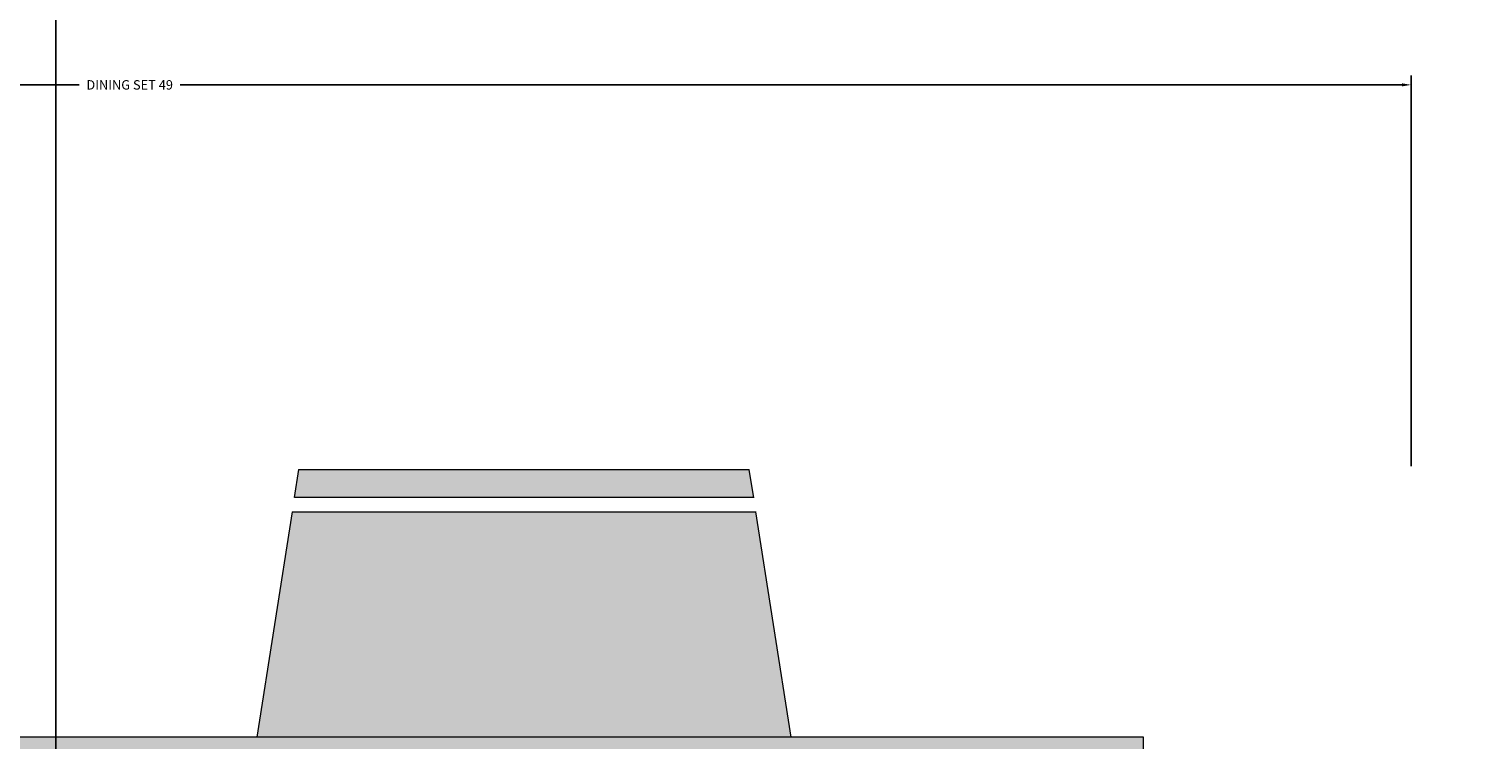
# Model space of a CAD drawing. Units: inches. Extents: x 2549 to 3108, y 1683 to 2362.
# Tile 14 of 30: x 2734 to 2762, y 2041 to 2055. Entities that reach past the tile are written whole.
import ezdxf

# ---------------------------------------------------------------- set-up
doc = ezdxf.new("R2010")
doc.units = ezdxf.units.IN
for name, color, linetype, lineweight in [('A-ANNO-DIMS', 2, 'Continuous', 18), ('A-FURN', 8, 'Continuous', 18), ('A-FURN-PATT', 9, 'Continuous', 13)]:
    doc.layers.add(name, color=color, linetype=linetype, lineweight=lineweight)
doc.layers.add('C-PKNG-VEHI-PATT', color=251, linetype='Continuous', lineweight=13, true_color=0x636466)
doc.layers.add('C-PVMT-PATT', color=9, linetype='Continuous', lineweight=13, true_color=0xc7c8ca)
doc.styles.get("Standard").update_dxf_attribs({"font": 'arial.ttf'})
doc.dimstyles.get("Standard").update_dxf_attribs({"dimtxt": 0.18, "dimasz": 0.18, "dimexe": 0.18, "dimexo": 0.0625, "dimgap": 0.09, "dimtad": 0, "dimtih": 1, "dimtoh": 1, "dimdec": 4, "dimzin": 0, "dimdsep": 46, "dimtxsty": 'Standard', "dimcen": 0.09, "dimadec": 0, "dimazin": 0, "dimtfac": 1, "dimtdec": 4, "dimtofl": 0, "dimtmove": 0, "dimatfit": 3, "dimfxl": 1, "dimtolj": 1, "dimtzin": 0, "dimarcsym": 0})

# ---------------------------------------------------------------- blocks, each defined once
blk = doc.blocks.new('Dining Set - 36 x 72 in.')
for p, q in [((6, 27.5), (5.8438, 26.50042)), ((6, 27.5), (22, 27.5)), ((22.1563, 26.49966), (22, 27.5)), ((22.1584, 26.5), (5.8466, 26.5)), ((5.7657, 26.00059), (4.5153, 17.99762)), ((5.7696, 26), (22.2392, 26)), ((23.4848, 17.99762), (22.2345, 25.99926)), ((36, 18), (-36, 18)), ((36, -18), (36, 18))]:
    blk.add_line(p, q)
blk = doc.blocks.new('*D20')
at = {"layer": 'A-ANNO-DIMS', "color": 0, "lineweight": -2, "transparency": 16777216}
for p, q in [((2711.514, 2046.346), (2711.514, 2053.826)), ((2760.597, 2046.346), (2760.597, 2053.826)), ((2711.694, 2053.646), (2735.087, 2053.646)), ((2760.417, 2053.646), (2737.025, 2053.646))]:
    blk.add_line(p, q, dxfattribs=at)
at = {"layer": 'A-ANNO-DIMS', "color": 0, "transparency": 16777216}
for points in [[(2711.694, 2053.676), (2711.694, 2053.616), (2711.514, 2053.646)], [(2760.417, 2053.676), (2760.417, 2053.616), (2760.597, 2053.646)]]:
    blk.add_solid(points, dxfattribs=at)
at = {"layer": 'Defpoints', "color": 0, "transparency": 16777216}
for p in [(2760.597, 2053.646), (2711.514, 2046.283), (2760.597, 2046.283)]:
    blk.add_point(p, dxfattribs=at)
at = {"layer": 'A-ANNO-DIMS', "color": 0, "transparency": 16777216, "insert": (2736.056, 2053.646), "char_height": 0.18, "attachment_point": 5}
blk.add_mtext('\\A1;DINING SET 49', dxfattribs=at)
blk = doc.blocks.new('*D43')
at = {"layer": 'A-ANNO-DIMS', "color": 0, "lineweight": -2, "transparency": 16777216}
for p, q in [((2734.643, 2080.461), (2734.643, 1683.444)), ((2806.643, 2080.461), (2806.643, 1683.444)), ((2734.823, 1683.624), (2770.425, 1683.624)), ((2806.463, 1683.624), (2770.86, 1683.624))]:
    blk.add_line(p, q, dxfattribs=at)
at = {"layer": 'A-ANNO-DIMS', "color": 0, "transparency": 16777216}
for points in [[(2734.823, 1683.654), (2734.823, 1683.594), (2734.643, 1683.624)], [(2806.463, 1683.654), (2806.463, 1683.594), (2806.643, 1683.624)]]:
    blk.add_solid(points, dxfattribs=at)
at = {"layer": 'Defpoints', "color": 0, "transparency": 16777216}
for p in [(2734.643, 2080.524), (2806.643, 2080.524), (2806.643, 1683.624)]:
    blk.add_point(p, dxfattribs=at)
at = {"layer": 'A-ANNO-DIMS', "color": 0, "transparency": 16777216, "insert": (2770.643, 1683.624), "char_height": 0.18, "attachment_point": 5}
blk.add_mtext('\\A1;72', dxfattribs=at)
blk = doc.blocks.new('*D59')
at = {"layer": 'A-ANNO-DIMS', "color": 0, "lineweight": -2, "transparency": 16777216}
for p, q in [((2680.978, 1761.586), (2680.978, 2362.323)), ((2786.158, 1761.586), (2786.158, 2362.323)), ((2681.158, 2362.143), (2733.112, 2362.143)), ((2785.978, 2362.143), (2734.023, 2362.143))]:
    blk.add_line(p, q, dxfattribs=at)
at = {"layer": 'A-ANNO-DIMS', "color": 0, "transparency": 16777216}
for points in [[(2681.158, 2362.173), (2681.158, 2362.113), (2680.978, 2362.143)], [(2785.978, 2362.173), (2785.978, 2362.113), (2786.158, 2362.143)]]:
    blk.add_solid(points, dxfattribs=at)
at = {"layer": 'Defpoints', "color": 0, "transparency": 16777216}
for p in [(2786.158, 2362.143), (2680.978, 1761.524), (2786.158, 1761.524)]:
    blk.add_point(p, dxfattribs=at)
at = {"layer": 'A-ANNO-DIMS', "color": 0, "transparency": 16777216, "insert": (2733.568, 2362.143), "char_height": 0.18, "attachment_point": 5}
blk.add_mtext('\\A1;105.18', dxfattribs=at)

msp = doc.modelspace()

# ---------------------------------------------------------------- hatches: boundary and pattern name
at = {"layer": 'A-FURN-PATT'}
h = msp.add_hatch(color=256, dxfattribs=at)
h.dxf.hatch_style = 1
h.paths.add_polyline_path([(2732.9458, 2045.4744), (2724.0631, 2045.4744), (2723.389, 2041.1594), (2733.6201, 2041.1594)])
h.paths.add_polyline_path([(2748.0481, 2045.4744), (2739.1654, 2045.4744), (2738.4912, 2041.1594), (2748.7223, 2041.1594)])
h.paths.add_polyline_path([(2747.9217, 2046.2834), (2739.2918, 2046.2834), (2739.2075, 2045.7441), (2748.006, 2045.7441)])
h.paths.add_polyline_path([(2732.8194, 2046.2834), (2724.1896, 2046.2834), (2724.1053, 2045.7441), (2732.9037, 2045.7441)])
h.paths.add_polyline_path([(2759.7877, 2035.8922), (2755.4728, 2036.5664), (2755.4728, 2026.3353), (2759.7877, 2027.0095)])
h.paths.add_polyline_path([(2760.5968, 2035.7658), (2760.0574, 2035.8501), (2760.0574, 2027.0516), (2760.5968, 2027.1359)])
h.paths.add_polyline_path([(2716.6384, 2036.5664), (2712.3235, 2035.8922), (2712.3235, 2027.0095), (2716.6384, 2026.3353)])
h.paths.add_polyline_path([(2733.6201, 2021.7423), (2723.389, 2021.7423), (2724.0631, 2017.4273), (2732.9458, 2017.4273)])
h.paths.add_polyline_path([(2748.7223, 2021.7423), (2738.4912, 2021.7423), (2739.1654, 2017.4273), (2748.0481, 2017.4273)])
h.paths.add_polyline_path([(2748.006, 2017.1576), (2739.2075, 2017.1576), (2739.2918, 2016.6183), (2747.9217, 2016.6183)])
h.paths.add_polyline_path([(2732.9037, 2017.1576), (2724.1053, 2017.1576), (2724.1896, 2016.6183), (2732.8194, 2016.6183)])
h.paths.add_polyline_path([(2712.0538, 2035.85), (2711.5145, 2035.7658), (2711.5145, 2027.1359), (2712.0538, 2027.0516)])
h = msp.add_hatch(color=256, dxfattribs=at)
h.dxf.hatch_style = 1
h.paths.add_polyline_path([(2744.8667, 2037.254), (2744.7754, 2037.3839), (2744.7125, 2037.4849), (2744.6595, 2037.5854), (2744.5963, 2037.7375), (2744.5695, 2037.9287), (2744.6003, 2038.0617), (2744.6406, 2038.148), (2744.7014, 2038.2298), (2744.7817, 2038.3053), (2744.8799, 2038.3724), (2744.9945, 2038.4289), (2745.1238, 2038.4728), (2745.2663, 2038.5019), (2745.4204, 2038.5142), (2745.5844, 2038.5076), (2745.7585, 2038.4805), (2745.9486, 2038.4342), (2746.1624, 2038.3705), (2746.4075, 2038.2913), (2746.6917, 2038.1983), (2747.0224, 2038.0936), (2747.4074, 2037.9788), (2747.8543, 2037.8558), (2748.3724, 2037.7256), (2748.9783, 2037.5851), (2749.69, 2037.4304), (2750.5258, 2037.2575), (2751.5038, 2037.0624), (2752.6422, 2036.8414), (2753.9591, 2036.5902), (2755.4728, 2036.3051), (2755.4728, 2039.002), (2754.0892, 2039.103), (2752.7721, 2039.2035), (2751.5251, 2039.303), (2750.3516, 2039.4009), (2749.255, 2039.4967), (2748.2388, 2039.5898), (2747.3063, 2039.6798), (2746.4609, 2039.7661), (2745.7045, 2039.8482), (2745.0321, 2039.9255), (2744.4371, 2039.9976), (2743.9129, 2040.0639), (2743.4531, 2040.1238), (2743.0509, 2040.1769), (2742.6998, 2040.2227), (2742.3932, 2040.2605), (2742.1251, 2040.29), (2741.8917, 2040.3111), (2741.69, 2040.3237), (2741.5167, 2040.3279), (2741.3687, 2040.3237), (2741.2428, 2040.3111), (2741.1359, 2040.29), (2741.0448, 2040.2605), (2740.9668, 2040.2227), (2740.9015, 2040.1776), (2740.8488, 2040.1262), (2740.8088, 2040.0695), (2740.7814, 2040.0085), (2740.7667, 2039.9445), (2740.7646, 2039.8783), (2740.7751, 2039.811), (2740.7978, 2039.7435), (2740.8306, 2039.6755), (2740.8707, 2039.6064), (2740.9155, 2039.5357), (2740.996, 2039.4111), (2741.0771, 2039.2637), (2741.1346, 2039.0945), (2741.1499, 2038.9139), (2741.1092, 2038.7391), (2741.0289, 2038.6239), (2740.9549, 2038.5525), (2740.8586, 2038.4895), (2740.733, 2038.4359), (2740.5693, 2038.3929), (2740.3593, 2038.3615), (2740.0946, 2038.3427), (2739.7666, 2038.3376), (2739.367, 2038.3473), (2738.8873, 2038.3727), (2738.3203, 2038.4145), (2737.6635, 2038.471), (2736.9156, 2038.5402), (2736.0753, 2038.6199), (2735.1412, 2038.7081), (2734.112, 2038.8025), (2732.9864, 2038.9012), (2731.7632, 2039.002), (2730.4376, 2039.1026), (2728.9922, 2039.2), (2727.4062, 2039.2911), (2725.6588, 2039.3728), (2723.7291, 2039.4418), (2721.5964, 2039.495), (2719.2397, 2039.5292), (2716.6384, 2039.5413), (2716.6384, 2036.8445), (2720.4266, 2036.9215), (2723.5572, 2036.9548), (2726.1183, 2036.9512), (2728.1983, 2036.9175), (2729.8853, 2036.8608), (2731.2677, 2036.7876), (2732.4336, 2036.705), (2733.4711, 2036.6198), (2734.4538, 2036.5375), (2735.3951, 2036.4589), (2736.2938, 2036.3835), (2737.1484, 2036.3108), (2737.9578, 2036.2401), (2738.7205, 2036.171), (2739.4353, 2036.103), (2740.1009, 2036.0355), (2740.7163, 2035.9683), (2741.2828, 2035.9027), (2741.8019, 2035.8403), (2742.2752, 2035.7826), (2742.7042, 2035.7313), (2743.0906, 2035.6878), (2743.4358, 2035.6539), (2743.7416, 2035.6309), (2744.0097, 2035.6203), (2744.243, 2035.6218), (2744.4448, 2035.6349), (2744.6181, 2035.659), (2744.7661, 2035.6937), (2744.892, 2035.7384), (2744.9989, 2035.7926), (2745.09, 2035.8557), (2745.1679, 2035.9271), (2745.2326, 2036.006), (2745.2836, 2036.0911), (2745.3204, 2036.1815), (2745.3424, 2036.2762), (2745.3492, 2036.374), (2745.3401, 2036.4739), (2745.3148, 2036.5748), (2745.2731, 2036.676), (2745.2178, 2036.7771), (2745.152, 2036.8782), (2745.0788, 2036.9794), (2745.0013, 2037.0805)])
h.paths.add_polyline_path([(2755.4728, 2036.3051), (2753.9591, 2036.5902), (2752.6422, 2036.8414), (2751.5038, 2037.0624), (2750.5258, 2037.2575), (2749.69, 2037.4304), (2748.9783, 2037.5851), (2748.3724, 2037.7256), (2747.8543, 2037.8558), (2747.4074, 2037.9788), (2747.0224, 2038.0936), (2746.6917, 2038.1983), (2746.4075, 2038.2913), (2746.1624, 2038.3705), (2745.9486, 2038.4342), (2745.7585, 2038.4805), (2745.5844, 2038.5076), (2745.4204, 2038.5142), (2745.2663, 2038.5019), (2745.1238, 2038.4728), (2744.9945, 2038.4289), (2744.8799, 2038.3724), (2744.7817, 2038.3053), (2744.7014, 2038.2298), (2744.6406, 2038.148), (2744.6003, 2038.0617), (2744.5794, 2037.9717), (2744.5765, 2037.8786), (2744.59, 2037.7828), (2744.6182, 2037.6849), (2744.6595, 2037.5854), (2744.7125, 2037.4849), (2744.7754, 2037.3839), (2744.8465, 2037.2827), (2744.9229, 2037.1816), (2745.0013, 2037.0805), (2745.1278, 2036.9154), (2745.2178, 2036.7771), (2745.2731, 2036.676), (2745.3148, 2036.5748), (2745.3401, 2036.4739), (2745.3492, 2036.374), (2745.3424, 2036.2762), (2745.3204, 2036.1815), (2745.2836, 2036.0911), (2745.2326, 2036.006), (2745.1679, 2035.9271), (2745.09, 2035.8557), (2744.9989, 2035.7926), (2744.892, 2035.7384), (2744.7661, 2035.6937), (2744.6181, 2035.659), (2744.4448, 2035.6349), (2744.243, 2035.6218), (2744.0097, 2035.6203), (2743.7416, 2035.6309), (2743.4358, 2035.6539), (2743.0906, 2035.6878), (2742.7042, 2035.7313), (2742.2752, 2035.7826), (2741.8019, 2035.8403), (2741.2828, 2035.9027), (2740.7163, 2035.9683), (2740.1009, 2036.0355), (2739.4353, 2036.103), (2738.7205, 2036.171), (2737.9578, 2036.2401), (2737.1484, 2036.3108), (2736.2938, 2036.3835), (2735.3951, 2036.4589), (2734.4538, 2036.5375), (2733.4711, 2036.6198), (2732.4336, 2036.705), (2731.2677, 2036.7876), (2729.8853, 2036.8608), (2728.1983, 2036.9175), (2726.1183, 2036.9512), (2723.5572, 2036.9548), (2720.4266, 2036.9215), (2716.6384, 2036.8445), (2716.6384, 2034.4174), (2719.4886, 2034.3283), (2721.9949, 2034.2608), (2724.1925, 2034.2112), (2726.1167, 2034.1758), (2727.8028, 2034.1509), (2729.2861, 2034.1329), (2730.602, 2034.1181), (2731.7856, 2034.1027), (2732.8685, 2034.0839), (2733.8666, 2034.0613), (2734.7919, 2034.0356), (2735.6567, 2034.0072), (2736.473, 2033.9768), (2737.253, 2033.9447), (2738.0088, 2033.9116), (2738.7525, 2033.878), (2739.493, 2033.8445), (2740.2273, 2033.812), (2740.9489, 2033.7816), (2741.6515, 2033.7544), (2742.3289, 2033.7314), (2742.9747, 2033.7137), (2743.5825, 2033.7022), (2744.1461, 2033.6982), (2744.6607, 2033.7024), (2745.1272, 2033.7151), (2745.5485, 2033.7361), (2745.9272, 2033.7656), (2746.2658, 2033.8036), (2746.567, 2033.8499), (2746.8334, 2033.9047), (2747.0677, 2033.9679), (2747.2728, 2034.0393), (2747.4525, 2034.1175), (2747.6113, 2034.201), (2747.7531, 2034.2881), (2747.8824, 2034.3774), (2748.0032, 2034.4672), (2748.1197, 2034.556), (2748.2363, 2034.6421), (2748.3567, 2034.7241), (2748.4828, 2034.8008), (2748.6163, 2034.8712), (2748.7588, 2034.9343), (2748.9118, 2034.9889), (2749.077, 2035.034), (2749.2558, 2035.0686), (2749.4499, 2035.0916), (2749.6603, 2035.1022), (2749.8861, 2035.1007), (2750.1254, 2035.0876), (2750.3769, 2035.0635), (2750.639, 2035.0288), (2750.91, 2034.9841), (2751.1884, 2034.93), (2751.4725, 2034.8668), (2751.7642, 2034.7949), (2752.0786, 2034.7123), (2752.4341, 2034.6172), (2752.849, 2034.5073), (2753.3419, 2034.3805), (2753.9313, 2034.2348), (2754.6354, 2034.068), (2755.4728, 2033.878)])
h.paths.add_polyline_path([(2755.4728, 2033.878), (2754.6354, 2034.068), (2753.9313, 2034.2348), (2753.3419, 2034.3805), (2752.849, 2034.5073), (2752.4341, 2034.6172), (2752.0786, 2034.7123), (2751.7642, 2034.7949), (2751.4725, 2034.8668), (2751.1884, 2034.93), (2750.91, 2034.9841), (2750.639, 2035.0288), (2750.3769, 2035.0635), (2750.1254, 2035.0876), (2749.8861, 2035.1007), (2749.6603, 2035.1022), (2749.4499, 2035.0916), (2749.2558, 2035.0686), (2749.077, 2035.034), (2748.9118, 2034.9889), (2748.7588, 2034.9343), (2748.6163, 2034.8712), (2748.4828, 2034.8008), (2748.3567, 2034.7241), (2748.2363, 2034.6421), (2748.1197, 2034.556), (2748.0032, 2034.4672), (2747.8824, 2034.3774), (2747.7531, 2034.2881), (2747.6113, 2034.201), (2747.4525, 2034.1175), (2747.2728, 2034.0393), (2747.0677, 2033.9679), (2746.8334, 2033.9047), (2746.567, 2033.8499), (2746.2658, 2033.8036), (2745.9272, 2033.7656), (2745.5485, 2033.7361), (2745.1272, 2033.7151), (2744.6607, 2033.7024), (2744.1461, 2033.6982), (2743.5825, 2033.7022), (2742.9747, 2033.7137), (2742.3289, 2033.7314), (2741.6515, 2033.7544), (2740.9489, 2033.7816), (2740.2273, 2033.812), (2739.493, 2033.8445), (2738.7525, 2033.878), (2738.0088, 2033.9116), (2737.253, 2033.9447), (2736.473, 2033.9768), (2735.6567, 2034.0072), (2734.7919, 2034.0356), (2733.8666, 2034.0613), (2732.8685, 2034.0839), (2731.7856, 2034.1027), (2730.602, 2034.1181), (2729.2861, 2034.1329), (2727.8028, 2034.1509), (2726.1167, 2034.1758), (2724.1925, 2034.2112), (2721.9949, 2034.2608), (2719.4886, 2034.3283), (2716.6384, 2034.4174), (2716.6384, 2030.9115), (2719.4477, 2031.0954), (2722.0216, 2031.2447), (2724.3773, 2031.363), (2726.5324, 2031.4537), (2728.5042, 2031.5201), (2730.3101, 2031.5657), (2731.9674, 2031.5939), (2733.4936, 2031.6082), (2734.9046, 2031.6115), (2736.2109, 2031.6057), (2737.4211, 2031.592), (2738.5446, 2031.5716), (2739.59, 2031.5461), (2740.5665, 2031.5165), (2741.4829, 2031.4843), (2742.3482, 2031.4509), (2743.1698, 2031.4174), (2743.9488, 2031.3855), (2744.6845, 2031.3568), (2745.3766, 2031.3329), (2746.0244, 2031.3152), (2746.6274, 2031.3055), (2747.1851, 2031.3052), (2747.697, 2031.316), (2748.1634, 2031.3388), (2748.5882, 2031.3722), (2748.9761, 2031.414), (2749.3319, 2031.4621), (2749.6603, 2031.5144), (2749.9661, 2031.5688), (2750.254, 2031.6233), (2750.5287, 2031.6756), (2750.7946, 2031.7239), (2751.0553, 2031.7669), (2751.314, 2031.8036), (2751.5737, 2031.8329), (2751.8375, 2031.8538), (2752.1088, 2031.8652), (2752.3906, 2031.8661), (2752.6861, 2031.8554), (2752.9965, 2031.8326), (2753.315, 2031.7999), (2753.633, 2031.7598), (2753.9418, 2031.7149), (2754.2327, 2031.6679), (2754.497, 2031.6215), (2754.7259, 2031.5782), (2754.911, 2031.5407), (2755.0467, 2031.5111), (2755.141, 2031.4888), (2755.2053, 2031.4728), (2755.2509, 2031.4621), (2755.2891, 2031.4556), (2755.3313, 2031.4523), (2755.3888, 2031.451), (2755.4728, 2031.4509)])
h.paths.add_polyline_path([(2743.9488, 2031.3855), (2743.1698, 2031.4174), (2742.3482, 2031.4509), (2741.4829, 2031.4843), (2740.5665, 2031.5165), (2739.59, 2031.5461), (2738.5446, 2031.5716), (2737.4211, 2031.592), (2736.2109, 2031.6057), (2734.9046, 2031.6115), (2733.4936, 2031.6082), (2731.9674, 2031.5939), (2730.3101, 2031.5657), (2728.5042, 2031.5201), (2726.5324, 2031.4537), (2724.3773, 2031.363), (2722.0216, 2031.2447), (2719.4477, 2031.0954), (2716.6384, 2030.9115), (2716.6384, 2027.945), (2721.3933, 2028.046), (2725.223, 2028.1465), (2728.2515, 2028.246), (2730.603, 2028.3439), (2732.4013, 2028.4397), (2733.7707, 2028.5328), (2734.8351, 2028.6228), (2735.7185, 2028.7091), (2736.5253, 2028.7912), (2737.2808, 2028.8692), (2737.9904, 2028.9429), (2738.6597, 2029.0125), (2739.2943, 2029.0778), (2739.8997, 2029.1389), (2740.4813, 2029.1958), (2741.0448, 2029.2484), (2741.5952, 2029.2967), (2742.1361, 2029.3397), (2742.6708, 2029.3764), (2743.2022, 2029.4058), (2743.7337, 2029.4266), (2744.2683, 2029.4381), (2744.8093, 2029.4389), (2745.3597, 2029.4282), (2745.9213, 2029.4053), (2746.4897, 2029.3713), (2747.0592, 2029.3279), (2747.6239, 2029.2765), (2748.1781, 2029.2189), (2748.716, 2029.1564), (2749.2317, 2029.0909), (2749.7196, 2029.0237), (2750.1754, 2028.9563), (2750.602, 2028.8892), (2751.0039, 2028.8226), (2751.3854, 2028.7568), (2751.7512, 2028.6921), (2752.1057, 2028.6287), (2752.4532, 2028.5668), (2752.7985, 2028.5068), (2753.1447, 2028.4496), (2753.4913, 2028.399), (2753.8363, 2028.3595), (2754.1778, 2028.3355), (2754.514, 2028.3315), (2754.8432, 2028.352), (2755.1634, 2028.4014), (2755.4728, 2028.4843), (2755.4728, 2031.4509), (2755.3151, 2031.4512), (2755.2429, 2031.4634), (2755.141, 2031.4888), (2755.0467, 2031.5111), (2754.911, 2031.5407), (2754.7259, 2031.5782), (2754.497, 2031.6215), (2754.2327, 2031.6679), (2753.9418, 2031.7149), (2753.633, 2031.7598), (2753.315, 2031.7999), (2752.9965, 2031.8326), (2752.6861, 2031.8554), (2752.3906, 2031.8661), (2752.1088, 2031.8652), (2751.8375, 2031.8538), (2751.5737, 2031.8329), (2751.314, 2031.8036), (2751.0553, 2031.7669), (2750.7946, 2031.7239), (2750.5287, 2031.6756), (2750.254, 2031.6233), (2749.9661, 2031.5688), (2749.6603, 2031.5144), (2749.3319, 2031.4621), (2748.9761, 2031.414), (2748.5882, 2031.3722), (2748.1634, 2031.3388), (2747.697, 2031.316), (2747.1851, 2031.3052), (2746.6274, 2031.3055), (2746.0244, 2031.3152), (2745.3766, 2031.3329), (2744.6845, 2031.3568)])
h.paths.add_polyline_path([(2755.4728, 2028.4843), (2755.1634, 2028.4014), (2754.8432, 2028.352), (2754.514, 2028.3315), (2754.1778, 2028.3355), (2753.8363, 2028.3595), (2753.4913, 2028.399), (2753.1447, 2028.4496), (2752.7985, 2028.5068), (2752.4532, 2028.5668), (2752.1057, 2028.6287), (2751.7512, 2028.6921), (2751.3854, 2028.7568), (2751.0039, 2028.8226), (2750.602, 2028.8892), (2750.1754, 2028.9563), (2749.7196, 2029.0237), (2749.2317, 2029.0909), (2748.716, 2029.1564), (2748.1781, 2029.2189), (2747.6239, 2029.2765), (2747.0592, 2029.3279), (2746.4897, 2029.3713), (2745.9213, 2029.4053), (2745.3597, 2029.4282), (2744.8093, 2029.4389), (2744.2683, 2029.4381), (2743.7337, 2029.4266), (2743.2022, 2029.4058), (2742.6708, 2029.3764), (2742.1361, 2029.3397), (2741.5952, 2029.2967), (2741.0448, 2029.2484), (2740.4813, 2029.1958), (2739.8997, 2029.1389), (2739.2943, 2029.0778), (2738.6597, 2029.0125), (2737.9904, 2028.9429), (2737.2808, 2028.8692), (2736.5253, 2028.7912), (2735.7185, 2028.7091), (2734.8351, 2028.6228), (2733.7707, 2028.5328), (2732.4013, 2028.4397), (2730.603, 2028.3439), (2728.2515, 2028.246), (2725.223, 2028.1465), (2721.3933, 2028.046), (2716.6384, 2027.945), (2716.6384, 2023.63), (2719.8271, 2023.719), (2722.5536, 2023.7853), (2724.8739, 2023.8315), (2726.8443, 2023.8604), (2728.5207, 2023.8745), (2729.9593, 2023.8765), (2731.2162, 2023.8691), (2732.3475, 2023.8548), (2733.4006, 2023.8359), (2734.3887, 2023.8133), (2735.3162, 2023.7876), (2736.1877, 2023.7593), (2737.0074, 2023.7288), (2737.7801, 2023.6968), (2738.5101, 2023.6637), (2739.2019, 2023.63), (2739.8611, 2023.5965), (2740.4973, 2023.5644), (2741.1215, 2023.5348), (2741.7443, 2023.5092), (2742.3766, 2023.4889), (2743.0291, 2023.4752), (2743.7127, 2023.4693), (2744.4383, 2023.4727), (2745.2212, 2023.4875), (2746.096, 2023.5194), (2747.1021, 2023.575), (2748.2785, 2023.6609), (2749.6645, 2023.7837), (2751.2994, 2023.9499), (2753.2224, 2024.1662), (2755.4728, 2024.4391)])
h.paths.add_polyline_path([(2755.4728, 2026.3269), (2754.9554, 2026.3329), (2754.418, 2026.3497), (2753.8658, 2026.3755), (2753.3041, 2026.4083), (2752.7382, 2026.4465), (2752.1734, 2026.4881), (2751.6149, 2026.5312), (2751.068, 2026.5741), (2750.5357, 2026.6151), (2750.0124, 2026.6538), (2749.4902, 2026.6898), (2748.9611, 2026.723), (2748.4173, 2026.753), (2747.8508, 2026.7795), (2747.2537, 2026.8024), (2746.6182, 2026.8213), (2745.9367, 2026.8359), (2745.2024, 2026.8452), (2744.4091, 2026.8482), (2743.5505, 2026.8438), (2742.6204, 2026.8309), (2741.6122, 2026.8087), (2740.5198, 2026.7758), (2739.3368, 2026.7314), (2738.0388, 2026.6748), (2736.5297, 2026.6071), (2734.695, 2026.5299), (2732.4205, 2026.4449), (2729.5919, 2026.3535), (2726.0949, 2026.2573), (2721.8152, 2026.1581), (2716.6384, 2026.0572), (2716.6384, 2023.63), (2719.8271, 2023.719), (2722.5536, 2023.7853), (2724.8739, 2023.8315), (2726.8443, 2023.8604), (2728.5207, 2023.8745), (2729.9593, 2023.8765), (2731.2162, 2023.8691), (2732.3475, 2023.8548), (2733.4006, 2023.8359), (2734.3887, 2023.8133), (2735.3162, 2023.7876), (2736.1877, 2023.7593), (2737.0074, 2023.7288), (2737.7801, 2023.6968), (2738.5101, 2023.6637), (2739.2019, 2023.63), (2739.8611, 2023.5965), (2740.4973, 2023.5644), (2741.1215, 2023.5348), (2741.7443, 2023.5092), (2742.3766, 2023.4889), (2743.0291, 2023.4752), (2743.7127, 2023.4693), (2744.4383, 2023.4727), (2745.2212, 2023.4875), (2746.096, 2023.5194), (2747.1021, 2023.575), (2748.2785, 2023.6609), (2749.6645, 2023.7837), (2751.2994, 2023.9499), (2753.2224, 2024.1662), (2755.4728, 2024.4391)], flags=17)
h.paths.add_polyline_path([(2740.4973, 2023.5644), (2739.8611, 2023.5965), (2739.2019, 2023.63), (2738.5101, 2023.6637), (2737.7801, 2023.6968), (2737.0074, 2023.7288), (2736.1877, 2023.7593), (2735.3162, 2023.7876), (2734.3887, 2023.8133), (2733.4006, 2023.8359), (2732.3475, 2023.8548), (2731.2162, 2023.8691), (2729.9593, 2023.8765), (2728.5207, 2023.8745), (2726.8443, 2023.8604), (2724.8739, 2023.8315), (2722.5536, 2023.7853), (2719.8271, 2023.719), (2716.6384, 2023.63), (2716.6384, 2021.7423), (2755.4728, 2021.7423), (2755.4728, 2024.4391), (2753.2224, 2024.1662), (2751.2994, 2023.9499), (2749.6645, 2023.7837), (2748.2785, 2023.6609), (2747.1021, 2023.575), (2746.096, 2023.5194), (2745.2212, 2023.4875), (2744.4383, 2023.4727), (2743.7127, 2023.4693), (2743.0291, 2023.4752), (2742.3766, 2023.4889), (2741.7443, 2023.5092), (2741.1215, 2023.5348)])
h.paths.add_polyline_path([(2741.1359, 2040.29), (2741.2428, 2040.3111), (2741.3687, 2040.3237), (2741.5167, 2040.3279), (2741.69, 2040.3237), (2741.8917, 2040.3111), (2742.1251, 2040.29), (2742.3932, 2040.2605), (2742.6998, 2040.2227), (2743.0509, 2040.1769), (2743.4531, 2040.1238), (2743.9129, 2040.0639), (2744.4371, 2039.9976), (2745.0321, 2039.9255), (2745.7045, 2039.8482), (2746.4609, 2039.7661), (2747.3063, 2039.6798), (2748.2388, 2039.5898), (2749.255, 2039.4967), (2750.3516, 2039.4009), (2751.5251, 2039.303), (2752.7721, 2039.2035), (2754.0892, 2039.103), (2755.4728, 2039.002), (2755.4728, 2041.1594), (2716.6384, 2041.1594), (2716.6384, 2039.5413), (2719.2397, 2039.5292), (2721.5964, 2039.495), (2723.7291, 2039.4418), (2725.6588, 2039.3728), (2727.4062, 2039.2911), (2728.9922, 2039.2), (2730.4376, 2039.1026), (2731.7632, 2039.002), (2732.9864, 2038.9012), (2734.112, 2038.8025), (2735.1412, 2038.7081), (2736.0753, 2038.6199), (2736.9156, 2038.5402), (2737.6635, 2038.471), (2738.3203, 2038.4145), (2738.8873, 2038.3727), (2739.367, 2038.3473), (2739.7666, 2038.3376), (2740.0946, 2038.3427), (2740.3593, 2038.3615), (2740.5693, 2038.3929), (2740.733, 2038.4359), (2740.8586, 2038.4895), (2740.9549, 2038.5525), (2741.0289, 2038.6239), (2741.0834, 2038.7021), (2741.12, 2038.7856), (2741.1403, 2038.8728), (2741.1458, 2038.962), (2741.1382, 2039.0518), (2741.1189, 2039.1406), (2741.0897, 2039.2267), (2741.0522, 2039.309), (2741.0089, 2039.3875), (2740.9625, 2039.4629), (2740.8772, 2039.5951), (2740.8072, 2039.7159), (2740.7635, 2039.8453), (2740.7677, 2039.9782), (2740.8229, 2040.1009), (2740.9289, 2040.2044), (2741.0448, 2040.2605)])
at = {"layer": 'C-PKNG-VEHI-PATT'}
h = msp.add_hatch(color=256, dxfattribs=at)
h.dxf.hatch_style = 1
edge = h.paths.add_edge_path()
edge.add_ellipse((2935.7258, 1791.964), major_axis=(-50.66, 0), ratio=0.8423039, start_angle=248.16505, end_angle=265.72258)
edge.add_line((2938.911, 1834.5507), (2925.8653, 1834.5507))
edge.add_ellipse((2929.0505, 1791.964), major_axis=(50.66, 0), ratio=0.8423039, start_angle=94.27742, end_angle=111.83495)
edge.add_line((2912.8508, 1832.3947), (2914.2044, 1822.2495))
edge.add_ellipse((2930.6538, 1783.1023), major_axis=(-49.3014, 0), ratio=0.8423039, start_angle=-85.12993, end_angle=-67.20809, ccw=False)
edge.add_line((2927.1247, 1824.5225), (2937.6516, 1824.5225))
edge.add_ellipse((2934.1225, 1783.1023), major_axis=(49.3014, 0), ratio=0.8423039, start_angle=67.20809, end_angle=85.12993, ccw=False)
edge.add_line((2950.5719, 1822.2495), (2951.9255, 1832.3947))
edge = h.paths.add_edge_path()
edge.add_ellipse((2903.4793, 1857.3351), major_axis=(-34.7979, 0), ratio=0.8423039, start_angle=180, end_angle=209.43857)
edge.add_ellipse((2961.297, 1857.3351), major_axis=(34.7979, 0), ratio=0.8423039, start_angle=150.56143, end_angle=180)
edge.add_line((2926.4991, 1857.3351), (2926.4991, 1843.7609))
edge.add_ellipse((2924.1251, 1844.3143), major_axis=(-0.2209, 3.9278), ratio=0.6038336, start_angle=89.00201, end_angle=253.65741, ccw=False)
edge.add_line((2921.7512, 1844.2222), (2921.7512, 1853.3975))
edge.add_line((2921.7512, 1853.3975), (2925.269, 1855.8484))
edge.add_ellipse((2925.4782, 1855.4931), major_axis=(0.4584, 0), ratio=0.8423039, start_angle=90, end_angle=134.48021, ccw=False)
edge.add_line((2925.4782, 1855.8792), (2926.4991, 1855.8792))
edge.add_line((2926.4991, 1855.8792), (2926.4991, 1857.3351))
edge.add_ellipse((2961.297, 1857.3351), major_axis=(34.7979, 0), ratio=0.8423039, start_angle=150.56143, end_angle=180, ccw=False)
edge.add_line((2932.3882, 1873.6501), (2932.3882, 1875.7801))
edge.add_ellipse((2932.3882, 1875.3939), major_axis=(0.4584, 0), ratio=0.8423039, start_angle=90, end_angle=127.93313)
edge.add_line((2932.1366, 1875.7167), (2928.5915, 1873.7564))
edge.add_ellipse((2899.9271, 2002.4692), major_axis=(155.4756, 0), ratio=0.84230387, start_angle=-80.743434, end_angle=-77.445067, ccw=False)
edge.add_ellipse((2949.4402, 1715.2151), major_axis=(-189.1422, 0), ratio=0.84230387, start_angle=-79.790461, end_angle=-77.555373)
edge.add_ellipse((3300.3614, 1852.5642), major_axis=(-386.1662, 0), ratio=0.84230387, start_angle=-2.863715, end_angle=2.198541)
edge.add_ellipse((2929.0505, 1792.5159), major_axis=(-55.6192, 0), ratio=0.8423039, start_angle=-85.91759, end_angle=-72.28005, ccw=False)
edge.add_line((2925.7129, 1839.2798), (2939.0634, 1839.2798))
edge.add_ellipse((2935.7258, 1792.5159), major_axis=(55.6192, 0), ratio=0.8423039, start_angle=72.28005, end_angle=85.91759, ccw=False)
edge.add_ellipse((2564.4149, 1852.5642), major_axis=(-386.1662, 0), ratio=0.84230387, start_angle=177.801459, end_angle=182.863715)
edge.add_ellipse((2915.3361, 1715.2151), major_axis=(189.1422, 0), ratio=0.84230387, start_angle=77.555373, end_angle=79.790461)
edge.add_ellipse((2964.8492, 2002.4692), major_axis=(-155.4756, 0), ratio=0.84230387, start_angle=77.445067, end_angle=80.743434, ccw=False)
edge.add_line((2936.1848, 1873.7564), (2932.6397, 1875.7167))
edge.add_ellipse((2932.3882, 1875.3939), major_axis=(0.4584, 0), ratio=0.8423039, start_angle=52.06687, end_angle=90)
edge.add_line((2932.3882, 1875.7801), (2932.3882, 1873.6501))
edge.add_ellipse((2903.4793, 1857.3351), major_axis=(-34.7979, 0), ratio=0.8423039, start_angle=180, end_angle=209.43857, ccw=False)
edge.add_line((2938.2772, 1857.3351), (2938.2772, 1855.8792))
edge.add_line((2938.2772, 1855.8792), (2939.4059, 1855.8792))
edge.add_ellipse((2939.2981, 1855.4931), major_axis=(-0.4584, 0), ratio=0.8423039, start_angle=225.51979, end_angle=270, ccw=False)
edge.add_line((2939.5903, 1855.7906), (2943.0251, 1853.3975))
edge.add_line((2943.0251, 1853.3975), (2943.0251, 1844.2222))
edge.add_ellipse((2940.6512, 1844.3143), major_axis=(0.2209, 3.9278), ratio=0.6038336, start_angle=106.34259, end_angle=270.99799, ccw=False)
edge.add_line((2938.2772, 1843.7609), (2938.2772, 1857.3351))
edge = h.paths.add_edge_path()
edge.add_ellipse((2932.3882, 1865.1973), major_axis=(91.081, 0), ratio=0.8423039, start_angle=256.401865, end_angle=283.598135, ccw=False)
edge.add_line((2914.2044, 1790.0239), (2914.2044, 1778.3622))
edge.add_ellipse((2932.3882, 1853.5356), major_axis=(91.081, 0), ratio=0.8423039, start_angle=256.401865, end_angle=283.598135)
edge.add_line((2950.5719, 1778.3622), (2950.5719, 1790.0239))
edge = h.paths.add_edge_path()
edge.add_ellipse((2948.7383, 1772.3145), major_axis=(1.8336, 0), ratio=0.8423039, start_angle=0, end_angle=90)
edge.add_line((2948.7383, 1773.859), (2916.038, 1773.859))
edge.add_ellipse((2916.038, 1772.3145), major_axis=(1.8336, 0), ratio=0.8423039, start_angle=90, end_angle=180)
edge.add_line((2914.2044, 1772.3145), (2914.2044, 1760.2558))
edge.add_line((2914.2044, 1760.2558), (2950.5719, 1760.2558))
edge.add_line((2950.5719, 1760.2558), (2950.5719, 1772.3145))
h.paths.add_polyline_path([(2748.8496, 2101.6383), (2798.148, 2101.6383), (2798.148, 2111.4248), (2748.8496, 2111.4248)], flags=9)
h.paths.add_polyline_path([(2685.2081, 2101.489), (2719.3253, 2101.489), (2719.3253, 2111.2819), (2685.2081, 2111.2819)], flags=9)
h.paths.add_polyline_path([(2814.6852, 1907.1328), (2847.8384, 1907.1328), (2847.8384, 1916.9258), (2814.6852, 1916.9258)], flags=9)
h.paths.add_polyline_path([(2814.3906, 1835.5864), (2848.0172, 1835.5864), (2848.0172, 1845.3794), (2814.3906, 1845.3794)], flags=9)
h.paths.add_polyline_path([(2800.5245, 1759.1674), (2853.7435, 1759.1674), (2853.7435, 1768.954), (2800.5245, 1768.954)], flags=9)
h.paths.add_polyline_path([(2972.4611, 1807.3305), (3015.3943, 1807.3305), (3015.3943, 1817.117), (2972.4611, 1817.117)], flags=9)
h.paths.add_polyline_path([(2902.3327, 1888.6731), (2937.9131, 1888.6731), (2937.9131, 1898.4661), (2902.3327, 1898.4661)], flags=9)
h.paths.add_polyline_path([(2712.1779, 1878.9039), (2754.1257, 1878.9039), (2754.1257, 1888.6904), (2712.1779, 1888.6904)], flags=9)
h.paths.add_polyline_path([(2614.0056, 2012.812), (2650.0251, 2012.812), (2650.0251, 2022.4371), (2614.0056, 2022.4371)], flags=9)
h.paths.add_polyline_path([(2713.3129, 2003.1645), (2747.4237, 2003.1645), (2747.4237, 2012.951), (2713.3129, 2012.951)], flags=9)
h.paths.add_polyline_path([(2950.1379, 2001.6934), (2982.2992, 2001.6934), (2982.2992, 2011.48), (2950.1379, 2011.48)], flags=9)
h.paths.add_polyline_path([(2940.864, 2238.5537), (2997.5066, 2238.5537), (2997.5066, 2248.3466), (2940.864, 2248.3466)], flags=9)
h.paths.add_polyline_path([(2821.5457, 2202.8348), (2855.663, 2202.8348), (2855.663, 2212.6278), (2821.5457, 2212.6278)], flags=9)
h.paths.add_polyline_path([(2661.8026, 2238.6249), (2718.4451, 2238.6249), (2718.4451, 2248.4179), (2661.8026, 2248.4179)], flags=9)
at = {"layer": 'C-PVMT-PATT'}
h = msp.add_hatch(color=256, dxfattribs=at)
h.dxf.hatch_style = 1
h.paths.add_polyline_path([(3067.6427, 2305.5237), (2605.6427, 2305.5237), (2605.6427, 2074.5237), (2629.6427, 2074.5237), (2629.6427, 2281.5237), (3043.6427, 2281.5237), (3043.6427, 1885.5237), (3043.6427, 1872.8745), (3031.1672, 1872.8745), (3031.1672, 1862.5731), (2995.8054, 1862.5731), (2995.8054, 1872.8745), (2983.1752, 1872.8745), (2983.1752, 1885.5237), (2881.6427, 1885.5237), (2881.6427, 1795.5237), (2751.0977, 1795.5237), (2751.0977, 1761.5237), (2786.1577, 1761.5237), (2786.1577, 1723.5237), (2881.84, 1723.5237), (2881.84, 1714.5237), (3067.6427, 1714.5237), (3067.6427, 1723.5237)])
edge = h.paths.add_edge_path(flags=16)
edge.add_ellipse((2949.4402, 1710.9683), major_axis=(-194.1014, 0), ratio=0.84230387, start_angle=-77.874034, end_angle=-76.219471, ccw=False)
edge.add_ellipse((2949.4402, 1715.2151), major_axis=(-189.1422, 0), ratio=0.84230387, start_angle=-79.790461, end_angle=-77.555373, ccw=False)
edge.add_ellipse((2899.9271, 2002.4692), major_axis=(155.4756, 0), ratio=0.84230387, start_angle=-80.743434, end_angle=-77.445067)
edge.add_line((2928.5915, 1873.7564), (2932.3882, 1875.8558))
edge.add_line((2932.3882, 1875.8558), (2936.1848, 1873.7564))
edge.add_ellipse((2964.8492, 2002.4692), major_axis=(-155.4756, 0), ratio=0.84230387, start_angle=77.445067, end_angle=80.743434)
edge.add_ellipse((2915.3361, 1715.2151), major_axis=(189.1422, 0), ratio=0.84230387, start_angle=77.555373, end_angle=79.790461, ccw=False)
edge.add_ellipse((2915.3361, 1710.9683), major_axis=(-194.1014, 0), ratio=0.84230387, start_angle=256.219471, end_angle=257.874034, ccw=False)
edge.add_ellipse((2628.2871, 1850.2612), major_axis=(-327.2532, 0), ratio=0.84230387, start_angle=182.17995, end_angle=183.650428, ccw=False)
edge.add_ellipse((2955.5637, 1861.9334), major_axis=(-0.9168, 0), ratio=0.8423039, start_angle=180, end_angle=270, ccw=False)
edge.add_line((2956.4805, 1862.3857), (2956.4805, 1846.4866))
edge.add_ellipse((2955.5637, 1846.939), major_axis=(-0.9168, 0), ratio=0.8423039, start_angle=90, end_angle=180, ccw=False)
edge.add_ellipse((-3607.0606, 1835.832), major_axis=(-6562.6242, 0), ratio=0.84230387, start_angle=179.61613322, end_angle=180.09022909, ccw=False)
edge.add_ellipse((2955.5637, 1791.0926), major_axis=(0.9168, 0), ratio=0.8423039, start_angle=0, end_angle=90, ccw=False)
edge.add_line((2956.4805, 1791.545), (2956.4805, 1775.6459))
edge.add_ellipse((2955.5637, 1776.0982), major_axis=(0.9168, 0), ratio=0.8423039, start_angle=270, end_angle=360, ccw=False)
edge.add_ellipse((-3607.0606, 1835.832), major_axis=(-6562.6242, 0), ratio=0.84230387, start_angle=179.3813568, end_angle=179.47172853, ccw=False)
edge.add_ellipse((2954.5907, 1763.8768), major_axis=(-1.3752, 0), ratio=0.8423039, start_angle=179.37176, end_angle=248.46476, ccw=False)
edge.add_ellipse((-3607.519, 1835.832), major_axis=(-6564.0409, 0), ratio=0.842303863, start_angle=179.35344594, end_angle=179.37176282, ccw=False)
edge.add_ellipse((2952.6829, 1761.8002), major_axis=(3.2503, 0), ratio=0.8423039, start_angle=-90, end_angle=-0.64655, ccw=False)
edge.add_line((2952.6829, 1759.0625), (2912.0934, 1759.0625))
edge.add_ellipse((2912.0934, 1761.8002), major_axis=(3.2503, 0), ratio=0.8423039, start_angle=180.64655, end_angle=270, ccw=False)
edge.add_ellipse((9472.2953, 1835.832), major_axis=(-6564.0409, 0), ratio=0.842303871, start_angle=0.62823722, end_angle=0.6465541, ccw=False)
edge.add_ellipse((2910.1856, 1763.8768), major_axis=(1.3752, 0), ratio=0.8423039, start_angle=111.53524, end_angle=180.62824, ccw=False)
edge.add_ellipse((9471.8369, 1835.832), major_axis=(-6562.6242, 0), ratio=0.84230387, start_angle=0.52827147, end_angle=0.6465541, ccw=False)
edge.add_ellipse((2909.2126, 1776.0982), major_axis=(-0.9168, 0), ratio=0.8423039, start_angle=0, end_angle=90, ccw=False)
edge.add_line((2908.2958, 1775.6459), (2908.2958, 1791.545))
edge.add_ellipse((2909.2126, 1791.0926), major_axis=(-0.9168, 0), ratio=0.8423039, start_angle=-90, end_angle=0, ccw=False)
edge.add_ellipse((9471.8369, 1835.832), major_axis=(-6562.6242, 0), ratio=0.84230387, start_angle=-0.09022909, end_angle=0.38386678, ccw=False)
edge.add_ellipse((2909.2126, 1846.939), major_axis=(-0.9168, 0), ratio=0.8423039, start_angle=0, end_angle=90, ccw=False)
edge.add_line((2908.2958, 1846.4866), (2908.2958, 1862.3857))
edge.add_ellipse((2909.2126, 1861.9334), major_axis=(0.9168, 0), ratio=0.8423039, start_angle=90, end_angle=180, ccw=False)
edge.add_ellipse((3236.4892, 1850.2612), major_axis=(327.2532, 0), ratio=0.84230387, start_angle=176.349572, end_angle=177.82005, ccw=False)
edge = h.paths.add_edge_path(flags=0)
edge.add_ellipse((2903.4793, 1857.3351), major_axis=(-34.7979, 0), ratio=0.8423039, start_angle=180, end_angle=209.43857, ccw=False)
edge.add_line((2938.2772, 1857.3351), (2938.2772, 1855.8792))
edge.add_line((2938.2772, 1855.8792), (2939.4631, 1855.8792))
edge.add_line((2939.4631, 1855.8792), (2943.0251, 1853.3975))
edge.add_line((2943.0251, 1853.3975), (2943.0251, 1844.2222))
edge.add_ellipse((2940.6512, 1844.3143), major_axis=(0.2209, 3.9278), ratio=0.6038336, start_angle=106.34259, end_angle=270.99799, ccw=False)
edge.add_line((2938.2772, 1843.7609), (2938.2772, 1857.3351))
edge.add_ellipse((2903.4793, 1857.3351), major_axis=(-34.7979, 0), ratio=0.8423039, start_angle=180, end_angle=209.43857)
edge.add_ellipse((2961.297, 1857.3351), major_axis=(34.7979, 0), ratio=0.8423039, start_angle=150.56143, end_angle=180)
edge.add_line((2926.4991, 1857.3351), (2926.4991, 1843.7609))
edge.add_ellipse((2924.1251, 1844.3143), major_axis=(-0.2209, 3.9278), ratio=0.6038336, start_angle=89.00201, end_angle=253.65741, ccw=False)
edge.add_line((2921.7512, 1844.2222), (2921.7512, 1853.3975))
edge.add_line((2921.7512, 1853.3975), (2925.3132, 1855.8792))
edge.add_line((2925.3132, 1855.8792), (2926.4991, 1855.8792))
edge.add_line((2926.4991, 1855.8792), (2926.4991, 1857.3351))
edge.add_ellipse((2961.297, 1857.3351), major_axis=(34.7979, 0), ratio=0.8423039, start_angle=150.56143, end_angle=180, ccw=False)
edge = h.paths.add_edge_path(flags=0)
edge.add_ellipse((2929.0505, 1791.964), major_axis=(50.66, 0), ratio=0.8423039, start_angle=94.27742, end_angle=111.83495, ccw=False)
edge.add_line((2925.8653, 1834.5507), (2938.911, 1834.5507))
edge.add_ellipse((2935.7258, 1791.964), major_axis=(-50.66, 0), ratio=0.8423039, start_angle=248.16505, end_angle=265.72258, ccw=False)
edge.add_line((2951.9255, 1832.3947), (2950.5719, 1822.2495))
edge.add_ellipse((2934.1225, 1783.1023), major_axis=(49.3014, 0), ratio=0.8423039, start_angle=67.20809, end_angle=85.12993)
edge.add_line((2937.6516, 1824.5225), (2927.1247, 1824.5225))
edge.add_ellipse((2930.6538, 1783.1023), major_axis=(-49.3014, 0), ratio=0.8423039, start_angle=-85.12993, end_angle=-67.20809)
edge.add_line((2914.2044, 1822.2495), (2912.8508, 1832.3947))
edge = h.paths.add_edge_path(flags=0)
edge.add_line((2910.1338, 1829.4651), (2912.6432, 1821.2711))
edge.add_ellipse((5203.7787, 1816.4367), major_axis=(-2291.1426, 0), ratio=0.84230387, start_angle=-0.1208974, end_angle=0.3640763)
edge.add_line((2912.7012, 1801.8782), (2910.3305, 1792.5698))
edge.add_ellipse((9471.8369, 1835.832), major_axis=(-6561.7074, 0), ratio=0.84230387, start_angle=0.05559431, end_angle=0.37776419, ccw=False)
edge = h.paths.add_edge_path(flags=0)
edge.add_ellipse((-3607.0606, 1835.832), major_axis=(6561.7074, 0), ratio=0.84230387, start_angle=-0.37776419, end_angle=-0.05559431, ccw=False)
edge.add_line((2954.4458, 1792.5698), (2952.0751, 1801.8782))
edge.add_ellipse((660.9976, 1816.4367), major_axis=(2291.1426, 0), ratio=0.84230387, start_angle=-0.3640763, end_angle=0.1208974)
edge.add_line((2952.1331, 1821.2711), (2954.6425, 1829.4651))
edge = h.paths.add_edge_path(flags=0)
edge.add_ellipse((2932.3882, 1865.1973), major_axis=(91.081, 0), ratio=0.8423039, start_angle=256.401865, end_angle=283.598135)
edge.add_line((2950.5719, 1790.0239), (2950.5719, 1778.3622))
edge.add_ellipse((2932.3882, 1853.5356), major_axis=(91.081, 0), ratio=0.8423039, start_angle=256.401865, end_angle=283.598135, ccw=False)
edge.add_line((2914.2044, 1778.3622), (2914.2044, 1790.0239))
edge = h.paths.add_edge_path(flags=0)
edge.add_line((2916.038, 1773.859), (2948.7383, 1773.859))
edge.add_ellipse((2948.7383, 1772.3145), major_axis=(1.8336, 0), ratio=0.8423039, start_angle=0, end_angle=90, ccw=False)
edge.add_line((2950.5719, 1772.3145), (2950.5719, 1760.2558))
edge.add_line((2950.5719, 1760.2558), (2914.2044, 1760.2558))
edge.add_line((2914.2044, 1760.2558), (2914.2044, 1772.3145))
edge.add_ellipse((2916.038, 1772.3145), major_axis=(1.8336, 0), ratio=0.8423039, start_angle=90, end_angle=180, ccw=False)
h.paths.add_polyline_path([(2629.6427, 1978.5237), (2605.6427, 1978.5237), (2605.6427, 1723.5237), (2629.6427, 1723.5237), (2629.6427, 1795.5237)], flags=17)
h.paths.add_polyline_path([(2800.5245, 1759.1674), (2853.7435, 1759.1674), (2853.7435, 1768.954), (2800.5245, 1768.954)], flags=24)
h.paths.add_polyline_path([(2972.4611, 1807.3305), (3015.3943, 1807.3305), (3015.3943, 1817.117), (2972.4611, 1817.117)], flags=24)

# ---------------------------------------------------------------- block references
at = {"layer": 'A-FURN', "xscale": 0.5393661791637867, "yscale": 0.5393661791637867, "zscale": 0.5393661791637867}
msp.add_blockref('Dining Set - 36 x 72 in.', (2736.0556, 2031.4509), dxfattribs=at)

# ---------------------------------------------------------------- dimensions: what is measured, and where the dimension line sits
at = {"layer": 'A-ANNO-DIMS'}
for base, p1, p2, override, picture, middle in [((2786.1577, 2362.1425), (2680.9778, 1761.5237), (2786.1577, 1761.5237), {"dimdec": 2, "dimlfac": 1, "dimrnd": 0, "dimzin": 0, "dimdsep": 46, "dimlunit": 2}, '*D59', (2733.5678, 2362.1425)), ((2806.6427, 1683.6237), (2734.6427, 2080.5237), (2806.6427, 2080.5237), {"dimdec": 0, "dimlfac": 1, "dimrnd": 0, "dimzin": 0, "dimdsep": 46, "dimlunit": 2}, '*D43', (2770.6427, 1683.6237))]:
    dim = msp.add_linear_dim(base=base, p1=p1, p2=p2, dimstyle='Standard', override=override, dxfattribs=at)
    dim.commit()
    dim.dimension.update_dxf_attribs({"geometry": picture, "text_midpoint": middle})
dim = msp.add_linear_dim(base=(2760.5968, 2053.6458), p1=(2711.5145, 2046.2834), p2=(2760.5968, 2046.2834), text='DINING SET <>', dimstyle='Standard', override={"dimdec": 0, "dimlfac": 1, "dimrnd": 0, "dimzin": 0, "dimdsep": 46, "dimlunit": 2}, dxfattribs=at)
dim.commit()
dim.dimension.update_dxf_attribs({"geometry": '*D20', "text_midpoint": (2736.0556, 2053.6458)})

doc.saveas('drawing.dxf')
